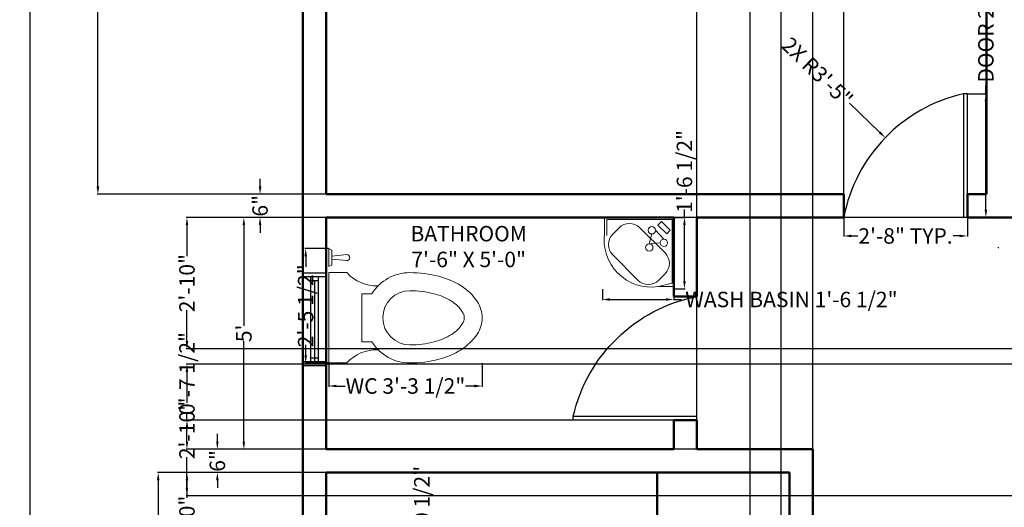
# Model space of a CAD drawing. Units: inches. Extents: x 2663 to 3147, y 140 to 736.
# Tile 4 of 6: x 2663 to 2918, y 425 to 551. Entities that reach past the tile are written whole.
import ezdxf

# ---------------------------------------------------------------- set-up
doc = ezdxf.new("R2010")
doc.units = ezdxf.units.IN
doc.header["$MEASUREMENT"] = 0
for name, color, linetype, lineweight in [('A-ANNO-DIMS', 2, 'Continuous', 18), ('A-AREA-IDEN', 3, 'Continuous', 25), ('A-DOOR', 3, 'Continuous', 25), ('A-FLOR-FIXT', 9, 'Continuous', 18), ('A-GLAZ', 4, 'Continuous', 25), ('A-WALL', 7, 'Continuous', 50)]:
    doc.layers.add(name, color=color, linetype=linetype, lineweight=lineweight)
doc.styles.get("Standard").update_dxf_attribs({"font": 'arial.ttf'})
doc.dimstyles.get("Standard").update_dxf_attribs({"dimtxt": 4, "dimasz": 2, "dimexe": 0.18, "dimexo": 0.0625, "dimgap": 0.09, "dimtad": 0, "dimdec": 0, "dimzin": 0, "dimdsep": 46, "dimlunit": 4, "dimtxsty": 'Standard', "dimcen": 0.09, "dimadec": 0, "dimazin": 0, "dimtfac": 1, "dimtdec": 0, "dimtofl": 0, "dimtmove": 0, "dimatfit": 3, "dimfxl": 1, "dimtolj": 1, "dimtzin": 0, "dimarcsym": 0})

# ---------------------------------------------------------------- blocks, each defined once
blk = doc.blocks.new('*D5')
at = {"layer": 'A-ANNO-DIMS', "color": 0, "lineweight": -2, "transparency": 16777216}
for p, q in [((2742.1, 434.32), (2698.54, 434.32)), ((2698.72, 432.32), (2698.72, 388.26)), ((2698.72, 340.32), (2698.72, 384.39)), ((2742.1, 338.32), (2698.54, 338.32))]:
    blk.add_line(p, q, dxfattribs=at)
at = {"layer": 'A-ANNO-DIMS', "color": 0, "transparency": 16777216}
for points in [[(2698.38, 432.32), (2699.05, 432.32), (2698.72, 434.32)], [(2698.38, 340.32), (2699.05, 340.32), (2698.72, 338.32)]]:
    blk.add_solid(points, dxfattribs=at)
at = {"layer": 'Defpoints', "color": 0, "transparency": 16777216}
for p in [(2698.72, 434.32), (2742.16, 434.32), (2742.16, 338.32)]:
    blk.add_point(p, dxfattribs=at)
at = {"layer": 'A-ANNO-DIMS', "color": 0, "transparency": 16777216, "insert": (2698.72, 386.32), "char_height": 4, "attachment_point": 5, "rotation": 90}
blk.add_mtext("\\A1;8'", dxfattribs=at)
blk = doc.blocks.new('DXFGVHBJKL')
for p, q in [((2908.16, 532.32), (2907.16, 532.32)), ((2907.16, 532.32), (2907.16, 500.32)), ((2908.16, 500.32), (2908.16, 532.32)), ((2908.16, 500.32), (2876.16, 500.32))]:
    blk.add_line(p, q)
blk.add_arc((2916.21, 492.54), 40.8, 102.812, 169.0067)
blk = doc.blocks.new('A$C756D1810')
at = {"linetype": 'ByBlock'}
for p, q in [((0, 0.6), (0, 0.5294)), ((0, 0.6), (0.3529, 0.6)), ((0.3529, 0.5294), (0.3529, 0.6)), ((0.3765, 0.6), (0.3824, 0.5882)), ((0.3765, 0.6), (0.4471, 0.6)), ((0.3824, 0.5882), (0.4412, 0.5882)), ((0.4, 0.5294), (0.4059, 0.5882)), ((0.4176, 0.5882), (0.4235, 0.5294)), ((0.4412, 0.5882), (0.4471, 0.6)), ((0.0824, 0.4706), (0.0824, 0.4316)), ((0.2706, 0.4706), (0.0824, 0.4706)), ((0.2706, 0.4706), (0.2706, 0.4316))]:
    blk.add_line(p, q, dxfattribs=at)
for centre, radius, start, end in [((-0.1078, 0.4118), 0.1596, 358.3378, 47.4896), ((0.4608, 0.4118), 0.1596, 132.5104, 181.6622), ((0.4118, 0.5294), 0.0118, 180, 0), ((0.1765, 0.2824), 0.1765, 122.231, 180), ((0.1765, 0.2824), 0.1765, 0, 57.769), ((0.1765, 0.2824), 0.1059, 0, 180), ((0.4502, 0.2824), 0.4502, 180, 194.5143), ((0.4502, 0.2824), 0.3796, 180, 194.5142), ((-0.0973, 0.2824), 0.3796, 345.4858, 360), ((-0.0973, 0.2824), 0.4502, 345.4857, 360), ((0.3152, 0.2474), 0.3108, 194.5143, 212.0054), ((0.3152, 0.2474), 0.2402, 194.5143, 212.0054), ((0.0377, 0.2474), 0.2402, 327.9946, 345.4857), ((0.0377, 0.2474), 0.3108, 327.9946, 345.4857), ((0.23, 0.1941), 0.1397, 212.0054, 236.4659), ((0.123, 0.1941), 0.1397, 303.5341, 327.9946), ((0.23, 0.1941), 0.2103, 212.0054, 236.4659), ((0.1765, 0.1134), 0.0428, 236.466, 270), ((0.1765, 0.1134), 0.0428, 270, 303.534), ((0.123, 0.1941), 0.2103, 303.5341, 327.9946), ((0.1765, 0.1134), 0.1134, 236.4659, 270), ((0.1765, 0.1134), 0.1134, 270, 303.5341)]:
    blk.add_arc(centre, radius, start, end, dxfattribs=at)
blk = doc.blocks.new('A$C017A17F4')
for p, q in [((0.45, 0.45), (0, 0.45)), ((0, 0.45), (0, 0.35)), ((0.45, 0), (0.45, 0.45)), ((0.3467, 0.3997), (0.3704, 0.4234)), ((0.4041, 0.3423), (0.3467, 0.3997)), ((0.3704, 0.4234), (0.4278, 0.366)), ((0.0533, 0.3414), (0.094, 0.3821)), ((0.2297, 0.3821), (0.3933, 0.2185)), ((0.4278, 0.366), (0.4041, 0.3423)), ((0.2168, 0.0421), (0.0533, 0.2056)), ((0.3933, 0.0827), (0.3526, 0.0421)), ((0.35, 0), (0.45, 0))]:
    blk.add_line(p, q)
at = {"ltscale": 10}
for p, q in [((0.4392, 0.4359), (0.0144, 0.4359)), ((0.0144, 0.4359), (0.0144, 0.3323)), ((0.4392, 0.4359), (0.4392, 0.0216)), ((0.3078, 0.342), (0.2911, 0.2778)), ((0.3317, 0.3659), (0.3861, 0.3086)), ((0.3622, 0.2847), (0.2911, 0.2778)), ((0.4392, 0.0216), (0.35, 0))]:
    blk.add_line(p, q, dxfattribs=at)
for centre in [(0.3078, 0.3659), (0.2911, 0.2539), (0.3861, 0.2847)]:
    blk.add_circle(centre, 0.0239, dxfattribs=at)
for centre, radius, start, end in [((0.1618, 0.3142), 0.096, 45, 135), ((0.3045, 0.3045), 0.3079, 171.50989, 278.49011), ((0.1212, 0.2735), 0.096, 135, 225), ((0.3254, 0.1506), 0.096, 315, 45), ((0.2847, 0.11), 0.096, 225, 315)]:
    blk.add_arc(centre, radius, start, end)
blk = doc.blocks.new('*D33')
at = {"layer": 'A-ANNO-DIMS', "color": 0, "lineweight": -2, "transparency": 16777216}
for p, q in [((2742.1, 500.32), (2720.71, 500.32)), ((2720.89, 498.32), (2720.89, 472.25)), ((2720.89, 442.32), (2720.89, 468.39)), ((2742.1, 440.32), (2720.71, 440.32))]:
    blk.add_line(p, q, dxfattribs=at)
at = {"layer": 'A-ANNO-DIMS', "color": 0, "transparency": 16777216}
for points in [[(2720.55, 498.32), (2721.22, 498.32), (2720.89, 500.32)], [(2720.55, 442.32), (2721.22, 442.32), (2720.89, 440.32)]]:
    blk.add_solid(points, dxfattribs=at)
at = {"layer": 'Defpoints', "color": 0, "transparency": 16777216}
for p in [(2720.89, 500.32), (2742.16, 500.32), (2742.16, 440.32)]:
    blk.add_point(p, dxfattribs=at)
at = {"layer": 'A-ANNO-DIMS', "color": 0, "transparency": 16777216, "insert": (2720.89, 470.32), "char_height": 4, "attachment_point": 5, "rotation": 90}
blk.add_mtext("\\A1;5'", dxfattribs=at)
blk = doc.blocks.new('*D34')
at = {"layer": 'A-ANNO-DIMS', "color": 0, "lineweight": -2, "transparency": 16777216}
for p, q in [((2714.03, 442.32), (2714.03, 444.32)), ((2736.1, 440.32), (2713.85, 440.32)), ((2736.1, 434.32), (2713.85, 434.32)), ((2714.03, 432.32), (2714.03, 430.32))]:
    blk.add_line(p, q, dxfattribs=at)
at = {"layer": 'A-ANNO-DIMS', "color": 0, "transparency": 16777216}
for points in [[(2713.7, 442.32), (2714.36, 442.32), (2714.03, 440.32)], [(2713.7, 432.32), (2714.36, 432.32), (2714.03, 434.32)]]:
    blk.add_solid(points, dxfattribs=at)
at = {"layer": 'Defpoints', "color": 0, "transparency": 16777216}
for p in [(2736.16, 440.32), (2714.03, 434.32), (2736.16, 434.32)]:
    blk.add_point(p, dxfattribs=at)
at = {"layer": 'A-ANNO-DIMS', "color": 0, "transparency": 16777216, "insert": (2714.03, 437.32), "char_height": 4, "attachment_point": 5, "rotation": 90}
blk.add_mtext('\\A1;6"', dxfattribs=at)
blk = doc.blocks.new('*D35')
at = {"layer": 'A-ANNO-DIMS', "color": 0, "lineweight": -2, "transparency": 16777216}
for p, q in [((2725.08, 508.32), (2725.08, 510.32)), ((2742.1, 506.32), (2724.9, 506.32)), ((2736.1, 500.32), (2724.9, 500.32)), ((2725.08, 498.32), (2725.08, 496.32))]:
    blk.add_line(p, q, dxfattribs=at)
at = {"layer": 'A-ANNO-DIMS', "color": 0, "transparency": 16777216}
for points in [[(2724.75, 508.32), (2725.42, 508.32), (2725.08, 506.32)], [(2724.75, 498.32), (2725.42, 498.32), (2725.08, 500.32)]]:
    blk.add_solid(points, dxfattribs=at)
at = {"layer": 'Defpoints', "color": 0, "transparency": 16777216}
for p in [(2725.08, 506.32), (2742.16, 506.32), (2736.16, 500.32)]:
    blk.add_point(p, dxfattribs=at)
at = {"layer": 'A-ANNO-DIMS', "color": 0, "transparency": 16777216, "insert": (2725.08, 503.32), "char_height": 4, "attachment_point": 5, "rotation": 90}
blk.add_mtext('\\A1;6"', dxfattribs=at)
blk = doc.blocks.new('*D36')
at = {"layer": 'A-ANNO-DIMS', "color": 0, "lineweight": -2, "transparency": 16777216}
for p, q in [((2742.1, 650.32), (2682.92, 650.32)), ((2683.1, 648.32), (2683.1, 581.62)), ((2683.1, 508.32), (2683.1, 575.03)), ((2742.1, 506.32), (2682.92, 506.32))]:
    blk.add_line(p, q, dxfattribs=at)
at = {"layer": 'A-ANNO-DIMS', "color": 0, "transparency": 16777216}
for points in [[(2682.77, 648.32), (2683.44, 648.32), (2683.1, 650.32)], [(2682.77, 508.32), (2683.44, 508.32), (2683.1, 506.32)]]:
    blk.add_solid(points, dxfattribs=at)
at = {"layer": 'Defpoints', "color": 0, "transparency": 16777216}
for p in [(2683.1, 650.32), (2742.16, 650.32), (2742.16, 506.32)]:
    blk.add_point(p, dxfattribs=at)
at = {"layer": 'A-ANNO-DIMS', "color": 0, "transparency": 16777216, "insert": (2683.1, 578.32), "char_height": 4, "attachment_point": 5, "rotation": 90}
blk.add_mtext("\\A1;12'", dxfattribs=at)
blk = doc.blocks.new('*D37')
at = {"layer": 'A-ANNO-DIMS', "color": 0, "lineweight": -2, "transparency": 16777216}
for p, q in [((2736.1, 656.32), (2665.31, 656.32)), ((2665.49, 654.32), (2665.49, 419.89)), ((2665.49, 178.32), (2665.49, 412.76)), ((2736.1, 176.32), (2665.31, 176.32))]:
    blk.add_line(p, q, dxfattribs=at)
at = {"layer": 'A-ANNO-DIMS', "color": 0, "transparency": 16777216}
for points in [[(2665.15, 654.32), (2665.82, 654.32), (2665.49, 656.32)], [(2665.15, 178.32), (2665.82, 178.32), (2665.49, 176.32)]]:
    blk.add_solid(points, dxfattribs=at)
at = {"layer": 'Defpoints', "color": 0, "transparency": 16777216}
for p in [(2665.49, 656.32), (2736.16, 656.32), (2736.16, 176.32)]:
    blk.add_point(p, dxfattribs=at)
at = {"layer": 'A-ANNO-DIMS', "color": 0, "transparency": 16777216, "insert": (2665.49, 416.32), "char_height": 4, "attachment_point": 5, "rotation": 90}
blk.add_mtext("\\A1;40'", dxfattribs=at)
blk = doc.blocks.new('*D39')
at = {"layer": 'A-ANNO-DIMS', "color": 0, "lineweight": -2, "transparency": 16777216}
for p, q in [((2912.96, 532.32), (2912.96, 534.32)), ((2908.22, 532.32), (2913.14, 532.32)), ((2912.96, 502.32), (2912.96, 530.32)), ((2908.22, 500.32), (2913.14, 500.32))]:
    blk.add_line(p, q, dxfattribs=at)
at = {"layer": 'A-ANNO-DIMS', "color": 0, "transparency": 16777216}
for points in [[(2912.63, 530.32), (2913.29, 530.32), (2912.96, 532.32)], [(2912.63, 502.32), (2913.29, 502.32), (2912.96, 500.32)]]:
    blk.add_solid(points, dxfattribs=at)
at = {"layer": 'Defpoints', "color": 0, "transparency": 16777216}
for p in [(2908.16, 532.32), (2912.96, 532.32), (2908.16, 500.32)]:
    blk.add_point(p, dxfattribs=at)
at = {"layer": 'A-ANNO-DIMS', "color": 0, "transparency": 16777216, "insert": (2912.96, 555.66), "char_height": 4, "attachment_point": 5, "rotation": 90}
blk.add_mtext('\\A1;DOOR 2\'-8" TYP.', dxfattribs=at)
blk = doc.blocks.new('*D40')
at = {"layer": 'A-ANNO-DIMS', "color": 0, "lineweight": -2, "transparency": 16777216}
for p, q in [((2876.16, 500.26), (2876.16, 495.34)), ((2908.16, 500.26), (2908.16, 495.34)), ((2878.16, 495.52), (2879.85, 495.52)), ((2906.16, 495.52), (2904.48, 495.52))]:
    blk.add_line(p, q, dxfattribs=at)
at = {"layer": 'A-ANNO-DIMS', "color": 0, "transparency": 16777216}
for points in [[(2878.16, 495.86), (2878.16, 495.19), (2876.16, 495.52)], [(2906.16, 495.86), (2906.16, 495.19), (2908.16, 495.52)]]:
    blk.add_solid(points, dxfattribs=at)
at = {"layer": 'Defpoints', "color": 0, "transparency": 16777216}
for p in [(2876.16, 500.32), (2908.16, 500.32), (2908.16, 495.52)]:
    blk.add_point(p, dxfattribs=at)
at = {"layer": 'A-ANNO-DIMS', "color": 0, "transparency": 16777216, "insert": (2892.16, 495.52), "char_height": 4, "attachment_point": 5}
blk.add_mtext('\\A1;2\'-8" TYP.', dxfattribs=at)
blk = doc.blocks.new('*D49')
at = {"layer": 'A-ANNO-DIMS', "color": 0, "lineweight": -2, "transparency": 16777216}
for p, q in [((2742.85, 462.6), (2742.85, 456.52)), ((2782.58, 462.6), (2782.58, 456.52)), ((2744.85, 456.7), (2747.14, 456.7)), ((2780.58, 456.7), (2778.3, 456.7))]:
    blk.add_line(p, q, dxfattribs=at)
at = {"layer": 'A-ANNO-DIMS', "color": 0, "transparency": 16777216}
for points in [[(2744.85, 457.04), (2744.85, 456.37), (2742.85, 456.7)], [(2780.58, 457.04), (2780.58, 456.37), (2782.58, 456.7)]]:
    blk.add_solid(points, dxfattribs=at)
at = {"layer": 'Defpoints', "color": 0, "transparency": 16777216}
for p in [(2742.85, 462.66), (2782.58, 462.66), (2742.85, 456.7)]:
    blk.add_point(p, dxfattribs=at)
at = {"layer": 'A-ANNO-DIMS', "color": 0, "transparency": 16777216, "insert": (2762.72, 456.7), "char_height": 4, "attachment_point": 5}
blk.add_mtext('\\A1;WC 3\'-3 1/2"', dxfattribs=at)
blk = doc.blocks.new('*D50')
at = {"layer": 'A-ANNO-DIMS', "color": 0, "lineweight": -2, "transparency": 16777216}
for p, q in [((2742.79, 492.26), (2736.71, 492.26)), ((2736.89, 490.26), (2736.89, 487.56)), ((2736.89, 464.66), (2736.89, 467.36)), ((2742.79, 462.66), (2736.71, 462.66))]:
    blk.add_line(p, q, dxfattribs=at)
at = {"layer": 'A-ANNO-DIMS', "color": 0, "transparency": 16777216}
for points in [[(2736.56, 490.26), (2737.23, 490.26), (2736.89, 492.26)], [(2736.56, 464.66), (2737.23, 464.66), (2736.89, 462.66)]]:
    blk.add_solid(points, dxfattribs=at)
at = {"layer": 'Defpoints', "color": 0, "transparency": 16777216}
for p in [(2736.89, 492.26), (2742.85, 492.26), (2742.85, 462.66)]:
    blk.add_point(p, dxfattribs=at)
at = {"layer": 'A-ANNO-DIMS', "color": 0, "transparency": 16777216, "insert": (2736.89, 477.46), "char_height": 4, "attachment_point": 5, "rotation": 90}
blk.add_mtext('\\A1;2\'-5 1/2"', dxfattribs=at)
blk = doc.blocks.new('*D51')
at = {"layer": 'A-ANNO-DIMS', "color": 0, "lineweight": -2, "transparency": 16777216}
for p, q in [((2813.69, 481.79), (2813.69, 478.9)), ((2832.16, 481.79), (2832.16, 478.9)), ((2815.69, 479.08), (2830.16, 479.08)), ((2832.16, 479.08), (2834.16, 479.08))]:
    blk.add_line(p, q, dxfattribs=at)
at = {"layer": 'A-ANNO-DIMS', "color": 0, "transparency": 16777216}
for points in [[(2815.69, 479.41), (2815.69, 478.75), (2813.69, 479.08)], [(2830.16, 479.41), (2830.16, 478.75), (2832.16, 479.08)]]:
    blk.add_solid(points, dxfattribs=at)
at = {"layer": 'Defpoints', "color": 0, "transparency": 16777216}
for p in [(2813.69, 481.85), (2832.16, 481.85), (2832.16, 479.08)]:
    blk.add_point(p, dxfattribs=at)
at = {"layer": 'A-ANNO-DIMS', "color": 0, "transparency": 16777216, "insert": (2862.63, 479.08), "char_height": 4, "attachment_point": 5}
blk.add_mtext('\\A1;WASH BASIN 1\'-6 1/2"', dxfattribs=at)
blk = doc.blocks.new('*D52')
at = {"layer": 'A-ANNO-DIMS', "color": 0, "lineweight": -2, "transparency": 16777216}
for p, q in [((2834.93, 500.32), (2834.93, 502.32)), ((2832.22, 500.32), (2835.11, 500.32)), ((2834.93, 483.85), (2834.93, 498.32)), ((2832.22, 481.85), (2835.11, 481.85))]:
    blk.add_line(p, q, dxfattribs=at)
at = {"layer": 'A-ANNO-DIMS', "color": 0, "transparency": 16777216}
for points in [[(2834.6, 498.32), (2835.27, 498.32), (2834.93, 500.32)], [(2834.6, 483.85), (2835.27, 483.85), (2834.93, 481.85)]]:
    blk.add_solid(points, dxfattribs=at)
at = {"layer": 'Defpoints', "color": 0, "transparency": 16777216}
for p in [(2832.16, 500.32), (2834.93, 500.32), (2832.16, 481.85)]:
    blk.add_point(p, dxfattribs=at)
at = {"layer": 'A-ANNO-DIMS', "color": 0, "transparency": 16777216, "insert": (2834.93, 512.2), "char_height": 4, "attachment_point": 5, "rotation": 90}
blk.add_mtext('\\A1;1\'-6 1/2"', dxfattribs=at)
blk = doc.blocks.new('*D53')
at = {"layer": 'A-ANNO-DIMS', "color": 0, "lineweight": -2, "transparency": 16777216}
for p, q in [((2766.95, 400.1), (2766.95, 402.1)), ((2763.37, 400.1), (2767.13, 400.1)), ((2766.95, 377.83), (2766.95, 398.1)), ((2763.37, 375.83), (2767.13, 375.83))]:
    blk.add_line(p, q, dxfattribs=at)
at = {"layer": 'A-ANNO-DIMS', "color": 0, "transparency": 16777216}
for points in [[(2766.62, 398.1), (2767.29, 398.1), (2766.95, 400.1)], [(2766.62, 377.83), (2767.29, 377.83), (2766.95, 375.83)]]:
    blk.add_solid(points, dxfattribs=at)
at = {"layer": 'Defpoints', "color": 0, "transparency": 16777216}
for p in [(2763.31, 400.1), (2766.95, 400.1), (2763.31, 375.83)]:
    blk.add_point(p, dxfattribs=at)
at = {"layer": 'A-ANNO-DIMS', "color": 0, "transparency": 16777216, "insert": (2766.95, 418.89), "char_height": 4, "attachment_point": 5, "rotation": 90}
blk.add_mtext('\\A1;HOB 2\'-0 1/2"', dxfattribs=at)
blk = doc.blocks.new('*D61')
at = {"layer": 'A-ANNO-DIMS', "color": 0, "lineweight": -2, "transparency": 16777216}
for p, q in [((2851.95, 276.84), (2851.95, 686.5)), ((2853.95, 686.32), (2857.98, 686.32)), ((2859.98, 276.84), (2859.98, 686.5)), ((2859.98, 686.32), (2861.98, 686.32))]:
    blk.add_line(p, q, dxfattribs=at)
at = {"layer": 'A-ANNO-DIMS', "color": 0, "transparency": 16777216}
for points in [[(2853.95, 686.66), (2853.95, 685.99), (2851.95, 686.32)], [(2857.98, 686.66), (2857.98, 685.99), (2859.98, 686.32)]]:
    blk.add_solid(points, dxfattribs=at)
at = {"layer": 'Defpoints', "color": 0, "transparency": 16777216}
for p in [(2859.98, 686.32), (2851.95, 276.78), (2859.98, 276.78)]:
    blk.add_point(p, dxfattribs=at)
at = {"layer": 'A-ANNO-DIMS', "color": 0, "transparency": 16777216, "insert": (2867.39, 686.32), "char_height": 4, "attachment_point": 5}
blk.add_mtext('\\A1;0\'-8"', dxfattribs=at)
blk = doc.blocks.new('*D75')
at = {"layer": 'A-ANNO-DIMS', "color": 0, "lineweight": -2, "transparency": 16777216}
for p, q in [((2742.16, 506.39), (2742.16, 686.5)), ((2744.16, 686.32), (2802.39, 686.32)), ((2874.16, 686.32), (2815.93, 686.32)), ((2876.16, 506.39), (2876.16, 686.5))]:
    blk.add_line(p, q, dxfattribs=at)
at = {"layer": 'A-ANNO-DIMS', "color": 0, "transparency": 16777216}
for points in [[(2744.16, 686.66), (2744.16, 685.99), (2742.16, 686.32)], [(2874.16, 686.66), (2874.16, 685.99), (2876.16, 686.32)]]:
    blk.add_solid(points, dxfattribs=at)
at = {"layer": 'Defpoints', "color": 0, "transparency": 16777216}
for p in [(2876.16, 686.32), (2742.16, 506.32), (2876.16, 506.32)]:
    blk.add_point(p, dxfattribs=at)
at = {"layer": 'A-ANNO-DIMS', "color": 0, "transparency": 16777216, "insert": (2809.16, 686.32), "char_height": 4, "attachment_point": 5}
blk.add_mtext('\\A1;11\'-2"', dxfattribs=at)
blk = doc.blocks.new('*D77')
at = {"layer": 'A-ANNO-DIMS', "color": 0, "lineweight": -2, "transparency": 16777216}
for p, q in [((2706.16, 447.86), (2706.16, 449.86)), ((2838.1, 447.86), (2705.98, 447.86)), ((2706.16, 442.32), (2706.16, 445.86)), ((2838.1, 440.32), (2705.98, 440.32))]:
    blk.add_line(p, q, dxfattribs=at)
at = {"layer": 'A-ANNO-DIMS', "color": 0, "transparency": 16777216}
for points in [[(2705.83, 445.86), (2706.49, 445.86), (2706.16, 447.86)], [(2705.83, 442.32), (2706.49, 442.32), (2706.16, 440.32)]]:
    blk.add_solid(points, dxfattribs=at)
at = {"layer": 'Defpoints', "color": 0, "transparency": 16777216}
for p in [(2706.16, 447.86), (2838.16, 447.86), (2838.16, 440.32)]:
    blk.add_point(p, dxfattribs=at)
at = {"layer": 'A-ANNO-DIMS', "color": 0, "transparency": 16777216, "insert": (2706.16, 459.93), "char_height": 4, "attachment_point": 5, "rotation": 90}
blk.add_mtext('\\A1;0\'-7 1/2"', dxfattribs=at)
blk = doc.blocks.new('*D78')
at = {"layer": 'A-ANNO-DIMS', "color": 0, "lineweight": -2, "transparency": 16777216}
for p, q in [((2838.16, 440.39), (2838.16, 686.5)), ((2840.16, 686.32), (2847.72, 686.32)), ((2866.16, 686.32), (2858.6, 686.32)), ((2868.16, 440.39), (2868.16, 686.5))]:
    blk.add_line(p, q, dxfattribs=at)
at = {"layer": 'A-ANNO-DIMS', "color": 0, "transparency": 16777216}
for points in [[(2840.16, 686.66), (2840.16, 685.99), (2838.16, 686.32)], [(2866.16, 686.66), (2866.16, 685.99), (2868.16, 686.32)]]:
    blk.add_solid(points, dxfattribs=at)
at = {"layer": 'Defpoints', "color": 0, "transparency": 16777216}
for p in [(2868.16, 686.32), (2838.16, 440.32), (2868.16, 440.32)]:
    blk.add_point(p, dxfattribs=at)
at = {"layer": 'A-ANNO-DIMS', "color": 0, "transparency": 16777216, "insert": (2853.16, 686.32), "char_height": 4, "attachment_point": 5}
blk.add_mtext('\\A1;2\'-6"', dxfattribs=at)
blk = doc.blocks.new('*D80')
at = {"layer": 'A-ANNO-DIMS', "color": 0, "lineweight": -2, "transparency": 16777216}
for p, q in [((2862.1, 434.32), (2705.98, 434.32)), ((2706.16, 432.32), (2706.16, 427.76)), ((2706.16, 412.32), (2706.16, 416.88)), ((2862.1, 410.32), (2705.98, 410.32))]:
    blk.add_line(p, q, dxfattribs=at)
at = {"layer": 'A-ANNO-DIMS', "color": 0, "transparency": 16777216}
for points in [[(2705.83, 432.32), (2706.49, 432.32), (2706.16, 434.32)], [(2705.83, 412.32), (2706.49, 412.32), (2706.16, 410.32)]]:
    blk.add_solid(points, dxfattribs=at)
at = {"layer": 'Defpoints', "color": 0, "transparency": 16777216}
for p in [(2706.16, 434.32), (2862.16, 434.32), (2862.16, 410.32)]:
    blk.add_point(p, dxfattribs=at)
at = {"layer": 'A-ANNO-DIMS', "color": 0, "transparency": 16777216, "insert": (2706.16, 422.32), "char_height": 4, "attachment_point": 5, "rotation": 90}
blk.add_mtext('\\A1;2\'-0"', dxfattribs=at)
blk = doc.blocks.new('*D85')
at = {"layer": 'A-ANNO-DIMS', "color": 0, "lineweight": -2, "transparency": 16777216}
for p, q in [((2964.1, 462.32), (2705.98, 462.32)), ((2706.16, 460.32), (2706.16, 452.32)), ((2706.16, 430.32), (2706.16, 438.33)), ((2964.1, 428.32), (2705.98, 428.32))]:
    blk.add_line(p, q, dxfattribs=at)
at = {"layer": 'A-ANNO-DIMS', "color": 0, "transparency": 16777216}
for points in [[(2705.83, 460.32), (2706.49, 460.32), (2706.16, 462.32)], [(2705.83, 430.32), (2706.49, 430.32), (2706.16, 428.32)]]:
    blk.add_solid(points, dxfattribs=at)
at = {"layer": 'Defpoints', "color": 0, "transparency": 16777216}
for p in [(2706.16, 462.32), (2964.16, 462.32), (2964.16, 428.32)]:
    blk.add_point(p, dxfattribs=at)
at = {"layer": 'A-ANNO-DIMS', "color": 0, "transparency": 16777216, "insert": (2706.16, 445.32), "char_height": 4, "attachment_point": 5, "rotation": 90}
blk.add_mtext('\\A1;2\'-10"', dxfattribs=at)
blk = doc.blocks.new('*D86')
at = {"layer": 'A-ANNO-DIMS', "color": 0, "lineweight": -2, "transparency": 16777216}
for p, q in [((2964.1, 500.32), (2705.98, 500.32)), ((2706.16, 498.32), (2706.16, 490.32)), ((2706.16, 468.32), (2706.16, 476.33)), ((2964.1, 466.32), (2705.98, 466.32))]:
    blk.add_line(p, q, dxfattribs=at)
at = {"layer": 'A-ANNO-DIMS', "color": 0, "transparency": 16777216}
for points in [[(2705.83, 498.32), (2706.49, 498.32), (2706.16, 500.32)], [(2705.83, 468.32), (2706.49, 468.32), (2706.16, 466.32)]]:
    blk.add_solid(points, dxfattribs=at)
at = {"layer": 'Defpoints', "color": 0, "transparency": 16777216}
for p in [(2706.16, 500.32), (2964.16, 500.32), (2964.16, 466.32)]:
    blk.add_point(p, dxfattribs=at)
at = {"layer": 'A-ANNO-DIMS', "color": 0, "transparency": 16777216, "insert": (2706.16, 483.32), "char_height": 4, "attachment_point": 5, "rotation": 90}
blk.add_mtext('\\A1;2\'-10"', dxfattribs=at)
blk = doc.blocks.new('*D88')
at = {"layer": 'A-ANNO-DIMS', "color": 0, "lineweight": -2, "transparency": 16777216}
for p, q in [((2877.7, 529.85), (2885.47, 522.32)), ((2916.12, 492.54), (2916.3, 492.54)), ((2916.21, 492.45), (2916.21, 492.63))]:
    blk.add_line(p, q, dxfattribs=at)
at = {"layer": 'A-ANNO-DIMS', "color": 0, "transparency": 16777216}
blk.add_solid([(2885.7, 522.56), (2885.24, 522.08), (2886.91, 520.93)], dxfattribs=at)
at = {"layer": 'Defpoints', "color": 0, "transparency": 16777216}
for p in [(2886.91, 520.93), (2916.21, 492.54)]:
    blk.add_point(p, dxfattribs=at)
at = {"layer": 'A-ANNO-DIMS', "color": 0, "transparency": 16777216, "insert": (2869.33, 537.96), "char_height": 4, "attachment_point": 5, "rotation": 315.9099}
blk.add_mtext('\\A1;2X R3\'-5"', dxfattribs=at)

msp = doc.modelspace()

# ---------------------------------------------------------------- linework, layer by layer
at = {"layer": 'A-GLAZ'}
for p, q in [((2736.16, 486), (2742.16, 486)), ((2736.16, 485), (2742.16, 485)), ((2738.16, 485), (2738.16, 463)), ((2740.16, 485), (2740.16, 463)), ((2738.16, 484), (2740.16, 484)), ((2739.16, 484), (2739.16, 463)), ((2738.16, 464), (2740.16, 464)), ((2736.16, 463), (2742.16, 463)), ((2736.16, 462), (2742.16, 462))]:
    msp.add_line(p, q, dxfattribs=at)
at = {"layer": 'A-WALL'}
for p, q in [((2736.16, 176.32), (2736.16, 656.32)), ((2742.16, 506.32), (2742.16, 650.32)), ((2913.16, 650.32), (2913.16, 506.32)), ((2742.16, 506.32), (2876.16, 506.32)), ((2876.16, 506.32), (2876.16, 500.32)), ((2908.16, 506.32), (2908.16, 500.32)), ((2908.16, 506.32), (2913.16, 506.32)), ((2742.16, 500.32), (2832.16, 500.32)), ((2742.16, 440.32), (2742.16, 500.32)), ((2832.16, 479.86), (2832.16, 500.32)), ((2838.16, 500.32), (2876.16, 500.32)), ((2838.16, 479.86), (2838.16, 500.32)), ((2908.16, 500.32), (2924.16, 500.32)), ((2838.16, 479.86), (2832.16, 479.86)), ((2832.16, 440.32), (2832.16, 447.86)), ((2832.16, 447.86), (2838.16, 447.86)), ((2838.16, 440.32), (2838.16, 447.86)), ((2742.16, 440.32), (2832.16, 440.32)), ((2838.16, 440.32), (2868.16, 440.32)), ((2868.16, 375.32), (2868.16, 440.32)), ((2742.16, 434.32), (2862.16, 434.32)), ((2742.16, 338.32), (2742.16, 434.32)), ((2827.83, 434.32), (2827.83, 410.32)), ((2862.16, 375.32), (2862.16, 434.32))]:
    msp.add_line(p, q, dxfattribs=at)

# ---------------------------------------------------------------- block references
at = {"layer": 'A-DOOR'}
msp.add_blockref('DXFGVHBJKL', (0, 0), dxfattribs=at)
at = {"layer": 'A-DOOR', "xscale": -1, "rotation": 89.9999999999992}
msp.add_blockref('DXFGVHBJKL', (3338.49, 3356.02), dxfattribs=at)
at = {"layer": 'A-FLOR-FIXT', "xscale": 39.7780062449713, "yscale": 39.7780062449713, "zscale": 39.7780062449713}
msp.add_blockref('A$C017A17F4', (2814.26, 482.42), dxfattribs=at)
at = {"layer": 'A-FLOR-FIXT', "xscale": 66.2133039807799, "yscale": 66.2133039807799, "zscale": 66.2133039807799, "rotation": 90}
msp.add_blockref('A$C756D1810', (2782.58, 462.66), dxfattribs=at)

# ---------------------------------------------------------------- texts
at = {"layer": 'A-AREA-IDEN', "insert": (2751.12, 498.11), "char_height": 4, "attachment_point": 1}
msp.add_mtext_dynamic_manual_height_columns('\\pxqc;BATHROOM\\P7\'-6" X 5\'-0"', width=55.9251, gutter_width=20, heights=[0], dxfattribs=at)

# ---------------------------------------------------------------- dimensions: what is measured, and where the dimension line sits
at = {"layer": 'A-ANNO-DIMS'}
for base, p1, p2, picture, middle in [((2876.16, 686.32), (2742.16, 506.32), (2876.16, 506.32), '*D75', (2809.16, 686.32)), ((2868.16, 686.32), (2838.16, 440.32), (2868.16, 440.32), '*D78', (2853.16, 686.32)), ((2859.98, 686.32), (2851.95, 276.78), (2859.98, 276.78), '*D61', (2867.39, 686.32))]:
    dim = msp.add_linear_dim(base=base, p1=p1, p2=p2, dimstyle='Standard', override={"dimdec": 1, "dimlfac": 1, "dimrnd": 0, "dimzin": 1, "dimdsep": 46, "dimlunit": 4, "dimfrac": 2}, dxfattribs=at)
    dim.commit()
    dim.dimension.update_dxf_attribs({"geometry": picture, "text_midpoint": middle})
for base, p1, p2, override, picture, middle in [((2665.49, 656.32), (2736.16, 176.32), (2736.16, 656.32), {"dimclrd": 0, "dimclre": 0, "dimclrt": 0}, '*D37', (2665.49, 416.32)), ((2683.1, 650.32), (2742.16, 506.32), (2742.16, 650.32), {"dimclrd": 0, "dimclre": 0, "dimclrt": 0}, '*D36', (2683.1, 578.32)), ((2834.93, 500.32), (2832.16, 481.85), (2832.16, 500.32), {"dimdec": 1, "dimrnd": 0, "dimzin": 1, "dimlunit": 4, "dimfrac": 2}, '*D52', (2834.93, 512.2)), ((2725.08, 506.32), (2736.16, 500.32), (2742.16, 506.32), {"dimclrd": 0, "dimclre": 0, "dimclrt": 0}, '*D35', (2725.08, 503.32)), ((2706.16, 500.32), (2964.16, 466.32), (2964.16, 500.32), {"dimdec": 1, "dimlfac": 1, "dimrnd": 0, "dimzin": 1, "dimdsep": 46, "dimlunit": 4, "dimfrac": 2}, '*D86', (2706.16, 483.32)), ((2720.89, 500.32), (2742.16, 440.32), (2742.16, 500.32), {"dimclrd": 0, "dimclre": 0, "dimclrt": 0}, '*D33', (2720.89, 470.32)), ((2736.89, 492.26), (2742.85, 462.66), (2742.85, 492.26), {"dimdec": 1, "dimrnd": 0, "dimzin": 1, "dimlunit": 4, "dimfrac": 2}, '*D50', (2736.89, 477.46)), ((2706.16, 447.86), (2838.16, 440.32), (2838.16, 447.86), {"dimdec": 1, "dimlfac": 1, "dimrnd": 0, "dimzin": 1, "dimdsep": 46, "dimlunit": 4, "dimfrac": 2}, '*D77', (2706.16, 459.93)), ((2706.16, 462.32), (2964.16, 428.32), (2964.16, 462.32), {"dimdec": 1, "dimlfac": 1, "dimrnd": 0, "dimzin": 1, "dimdsep": 46, "dimlunit": 4, "dimfrac": 2}, '*D85', (2706.16, 445.32)), ((2714.03, 434.32), (2736.16, 440.32), (2736.16, 434.32), {"dimclrd": 0, "dimclre": 0, "dimclrt": 0}, '*D34', (2714.03, 437.32)), ((2698.72, 434.32), (2742.16, 338.32), (2742.16, 434.32), {"dimclrd": 0, "dimclre": 0, "dimclrt": 0}, '*D5', (2698.72, 386.32)), ((2706.16, 434.32), (2862.16, 410.32), (2862.16, 434.32), {"dimdec": 1, "dimlfac": 1, "dimrnd": 0, "dimzin": 1, "dimdsep": 46, "dimlunit": 4, "dimfrac": 2}, '*D80', (2706.16, 422.32))]:
    dim = msp.add_linear_dim(base=base, p1=p1, p2=p2, angle=90, dimstyle='Standard', override=override, dxfattribs=at)
    dim.commit()
    dim.dimension.update_dxf_attribs({"geometry": picture, "text_midpoint": middle})
for base, p1, p2, angle, text, picture, middle in [((2912.96, 532.32), (2908.16, 500.32), (2908.16, 532.32), 90, 'DOOR <> TYP.', '*D39', (2912.96, 555.66)), ((2742.85, 456.7), (2782.58, 462.66), (2742.85, 462.66), 180, 'WC <>', '*D49', (2762.72, 456.7)), ((2766.95, 400.1), (2763.31, 375.83), (2763.31, 400.1), 90, 'HOB <>', '*D53', (2766.95, 418.89))]:
    dim = msp.add_linear_dim(base=base, p1=p1, p2=p2, angle=angle, text=text, dimstyle='Standard', override={"dimdec": 1, "dimrnd": 0, "dimzin": 1, "dimlunit": 4, "dimfrac": 2}, dxfattribs=at)
    dim.commit()
    dim.dimension.update_dxf_attribs({"geometry": picture, "text_midpoint": middle})
dim = msp.add_radius_dim(center=(2916.21, 492.54), mpoint=(2886.91, 520.93), text='2X <>', dimstyle='Standard', override={"dimdec": 1, "dimlfac": 1, "dimrnd": 0, "dimzin": 1, "dimdsep": 46, "dimlunit": 4, "dimfrac": 2}, dxfattribs=at)
dim.commit()
dim.dimension.update_dxf_attribs({"geometry": '*D88', "text_midpoint": (2869.33, 537.96), "dimtype": 164})
for base, p1, p2, text, picture, middle in [((2908.16, 495.52), (2876.16, 500.32), (2908.16, 500.32), '<> TYP.', '*D40', (2892.16, 495.52)), ((2832.16, 479.08), (2813.69, 481.85), (2832.16, 481.85), 'WASH BASIN <>', '*D51', (2862.63, 479.08))]:
    dim = msp.add_linear_dim(base=base, p1=p1, p2=p2, text=text, dimstyle='Standard', override={"dimdec": 1, "dimrnd": 0, "dimzin": 1, "dimlunit": 4, "dimfrac": 2}, dxfattribs=at)
    dim.commit()
    dim.dimension.update_dxf_attribs({"geometry": picture, "text_midpoint": middle})

doc.saveas('drawing.dxf')
